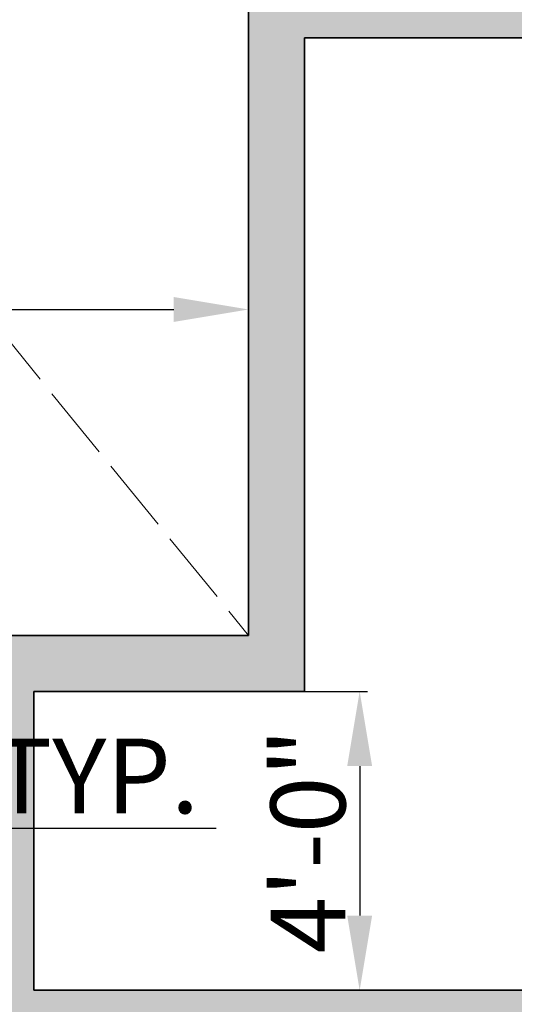
# Model space of a CAD drawing. Units: inches. Extents: x 2083 to 3317, y 1141 to 2115.
# Tile 88 of 256: x 2382 to 2462, y 1419 to 1577. Entities that reach past the tile are written whole.
import ezdxf

# ---------------------------------------------------------------- set-up
doc = ezdxf.new("R2010")
doc.units = ezdxf.units.IN
doc.linetypes.add('ACAD_ISO02W100', pattern=[15, 12, -3])
for name, color, linetype, lineweight in [('A-ANNO-DIMS', 2, 'Continuous', 18), ('A-FLOR-OPEN', 8, 'ACAD_ISO02W100', 13), ('A-WALL', 7, 'Continuous', 35)]:
    doc.layers.add(name, color=color, linetype=linetype, lineweight=lineweight)
doc.layers.add('A-WALL-PATT', color=251, linetype='Continuous', lineweight=13, true_color=0x636466)
doc.styles.get("Standard").update_dxf_attribs({"font": 'arial.ttf'})
doc.dimstyles.new('ISO-25', dxfattribs={"dimtxt": 12, "dimasz": 12, "dimexe": 1.25, "dimexo": 0.625, "dimtad": 1, "dimlunit": 3, "dimtxsty": 'Standard', "dimcen": 2.5, "dimadec": 0, "dimazin": 0, "dimtfac": 1, "dimtmove": 0, "dimatfit": 3, "dimfxl": 1, "dimarcsym": 0})

# ---------------------------------------------------------------- blocks, each defined once
blk = doc.blocks.new('*D30')
at = {"layer": 'A-ANNO-DIMS', "color": 0, "lineweight": -2, "transparency": 16777216}
for p, q in [((2240.02, 1445.27), (2240.02, 1448.05)), ((2254.33, 1445.27), (2254.33, 1448.05)), ((2228.02, 1446.8), (2216.02, 1446.8)), ((2240.02, 1446.8), (2254.33, 1446.8)), ((2266.33, 1446.8), (2413.76, 1446.8))]:
    blk.add_line(p, q, dxfattribs=at)
at = {"layer": 'A-ANNO-DIMS', "color": 0, "transparency": 16777216}
for points in [[(2228.02, 1448.8), (2228.02, 1444.8), (2240.02, 1446.8)], [(2266.33, 1448.8), (2266.33, 1444.8), (2254.33, 1446.8)]]:
    blk.add_solid(points, dxfattribs=at)
at = {"layer": 'Defpoints', "color": 0, "transparency": 16777216}
for p in [(2254.33, 1446.8), (2240.02, 1444.65), (2254.33, 1444.65)]:
    blk.add_point(p, dxfattribs=at)
at = {"layer": 'A-ANNO-DIMS', "color": 0, "transparency": 16777216, "insert": (2346.05, 1453.63), "char_height": 12, "attachment_point": 5}
blk.add_mtext('WC 1\'-2 1/2" TYP.', dxfattribs=at)
blk = doc.blocks.new('*D45')
at = {"layer": 'A-ANNO-DIMS', "color": 0, "lineweight": -2, "transparency": 16777216}
for p, q in [((2235.96, 1478.39), (2235.96, 1531.36)), ((2418.96, 1478.39), (2418.96, 1531.36)), ((2247.96, 1530.11), (2406.96, 1530.11))]:
    blk.add_line(p, q, dxfattribs=at)
at = {"layer": 'A-ANNO-DIMS', "color": 0, "transparency": 16777216}
for points in [[(2247.96, 1532.11), (2247.96, 1528.11), (2235.96, 1530.11)], [(2406.96, 1532.11), (2406.96, 1528.11), (2418.96, 1530.11)]]:
    blk.add_solid(points, dxfattribs=at)
at = {"layer": 'Defpoints', "color": 0, "transparency": 16777216}
for p in [(2418.96, 1530.11), (2235.96, 1477.76), (2418.96, 1477.76)]:
    blk.add_point(p, dxfattribs=at)
at = {"layer": 'A-ANNO-DIMS', "color": 0, "transparency": 16777216, "insert": (2327.46, 1536.87), "char_height": 12, "attachment_point": 5}
blk.add_mtext('15\'-3"', dxfattribs=at)
blk = doc.blocks.new('*D63')
at = {"layer": 'A-ANNO-DIMS', "color": 0, "lineweight": -2, "transparency": 16777216}
for p, q in [((2385.08, 1468.76), (2438.06, 1468.76)), ((2436.81, 1456.76), (2436.81, 1432.76)), ((2385.08, 1420.76), (2438.06, 1420.76))]:
    blk.add_line(p, q, dxfattribs=at)
at = {"layer": 'A-ANNO-DIMS', "color": 0, "transparency": 16777216}
for points in [[(2434.81, 1456.76), (2438.81, 1456.76), (2436.81, 1468.76)], [(2434.81, 1432.76), (2438.81, 1432.76), (2436.81, 1420.76)]]:
    blk.add_solid(points, dxfattribs=at)
at = {"layer": 'Defpoints', "color": 0, "transparency": 16777216}
for p in [(2384.46, 1468.76), (2384.46, 1420.76), (2436.81, 1420.76)]:
    blk.add_point(p, dxfattribs=at)
at = {"layer": 'A-ANNO-DIMS', "color": 0, "transparency": 16777216, "insert": (2430.06, 1444.76), "char_height": 12, "attachment_point": 5, "rotation": 90}
blk.add_mtext('4\'-0"', dxfattribs=at)

msp = doc.modelspace()

# ---------------------------------------------------------------- hatches: boundary and pattern name
at = {"layer": 'A-WALL-PATT'}
h = msp.add_hatch(color=256, dxfattribs=at)
h.dxf.hatch_style = 1
h.paths.add_polyline_path([(3126.96, 2020.761), (2748.96, 2020.761), (2604.96, 2020.761), (2226.96, 2020.761), (2226.96, 1702.761), (2466.96, 1702.761), (2466.96, 1582.761), (2418.96, 1582.761), (2418.96, 1477.761), (2226.96, 1477.761), (2226.96, 1263.261), (2544.96, 1263.261), (2544.96, 1411.761), (2604.96, 1411.761), (2685.96, 1411.761), (2685.96, 1420.761), (2604.96, 1420.761), (2604.96, 1573.761), (2604.96, 1702.761), (2604.96, 2011.761), (2748.96, 2011.761), (2748.96, 1702.761), (2862.96, 1702.761), (2862.96, 1621.761), (2871.96, 1621.761), (2871.96, 1702.761), (2883.96, 1702.761), (2883.96, 1706.939, -0.0264593), (2883.96, 1711.761), (2757.96, 1711.761), (2757.96, 1807.761), (2787.96, 1807.761), (2787.96, 1812.261), (2757.96, 1812.261), (2757.96, 2011.761), (2877.96, 2011.761), (2877.96, 1812.261), (2847.96, 1812.261), (2847.96, 1807.761), (2889.836, 1807.761), (2889.836, 1812.261), (2882.46, 1812.261), (2882.46, 2011.761), (3117.96, 2011.761), (3117.96, 1812.261), (2937.836, 1812.261), (2937.836, 1807.761), (2995.71, 1807.761), (2995.71, 1796.118), (3000.21, 1796.118), (3000.21, 1807.761), (3117.96, 1807.761), (3117.96, 1711.761), (3000.21, 1711.761), (3000.21, 1760.118), (2998.573, 1760.118, -0.020711), (2995.71, 1760.118), (2995.71, 1711.761), (2931.96, 1711.761), (2931.96, 1702.761), (3126.96, 1702.761)])
h.paths.add_polyline_path([(2471.46, 2011.761), (2471.46, 1810.011), (2462.717, 1810.011), (2462.717, 1805.511), (2505.96, 1805.511), (2505.96, 1810.011), (2475.96, 1810.011), (2475.96, 2011.761), (2595.96, 2011.761), (2595.96, 1810.011), (2565.96, 1810.011), (2565.96, 1805.511), (2595.96, 1805.511), (2595.96, 1711.761), (2235.96, 1711.761), (2235.96, 1805.511), (2353.71, 1805.511), (2353.71, 1796.054), (2358.21, 1796.054), (2358.21, 1805.511), (2414.717, 1805.511), (2414.717, 1810.011), (2235.96, 1810.011), (2235.96, 2011.761)], flags=16)
h.paths.add_polyline_path([(2270.205, 1994.61), (2270.205, 1970.61), (2246.205, 1970.61), (2246.205, 1994.61)], flags=0)
edge = h.paths.add_edge_path(flags=0)
edge.add_ellipse((2332.027, 1899.798), major_axis=(-3.043, 3.043), ratio=0.1682525, start_angle=-161.33217, end_angle=-156.30711, ccw=False)
edge.add_ellipse((2333.082, 1898.744), major_axis=(-1.055, 1.055), ratio=0.4535321, start_angle=-123.37102, end_angle=-94.15911)
edge = h.paths.add_edge_path(flags=0)
edge.add_ellipse((2332.027, 1968.876), major_axis=(3.043, 3.043), ratio=0.1682525, start_angle=18.66783, end_angle=23.69289)
edge.add_spline(control_points=[(2332.926, 1970.691), (2332.227, 1970.336), (2330.894, 1969.659), (2328.413, 1970.932), (2327.204, 1967.749), (2324.71, 1969.956), (2322.533, 1967.012), (2320.013, 1971.296), (2317.68, 1968.158), (2316.041, 1967.102), (2315.427, 1966.81)], knot_values=[0, 0, 0, 0, 2.2670587, 4.3245589, 6.6855835, 8.8786411, 11.121502, 14.300359, 17.7552837, 19.732645, 19.732645, 19.732645, 19.732645], degree=3, periodic=0)
edge.add_ellipse((2332.027, 1968.876), major_axis=(3.043, 3.043), ratio=0.1682525, start_angle=18.66783, end_angle=23.69289, ccw=False)
edge.add_ellipse((2333.082, 1969.931), major_axis=(1.055, 1.055), ratio=0.4535321, start_angle=56.62898, end_angle=85.84089, ccw=False)
edge = h.paths.add_edge_path(flags=0)
edge.add_spline(control_points=[(2296.428, 1967.988), (2293.628, 1965.336), (2287.704, 1959.727), (2299.744, 1949.996), (2294.533, 1935.669), (2290.573, 1920.604), (2293.394, 1909.974), (2296.185, 1904.967)], knot_values=[0.0991853, 0.0991853, 0.0991853, 0.0991853, 0.3453009, 0.6198217, 0.9826526, 1.3860932, 1.8105546, 1.8105546, 1.8105546, 1.8105546], degree=3, periodic=0)
edge.add_spline(control_points=[(2296.185, 1904.967), (2297.384, 1902.619), (2298.001, 1901.949), (2298.553, 1901.468)], knot_values=[0.0062457, 0.0062457, 0.0062457, 0.0062457, 0.0554759, 0.0554759, 0.0554759, 0.0554759], degree=3, periodic=0)
edge.add_spline(control_points=[(2298.553, 1901.468), (2297.259, 1900.923), (2295.225, 1900.232), (2293.06, 1900.614), (2292.101, 1900.788), (2292.09, 1900.791)], knot_values=[0.3128349, 0.3128349, 0.3128349, 0.3128349, 0.4017797, 0.4749867, 0.4759027, 0.4759027, 0.4759027, 0.4759027], degree=3, periodic=0)
edge.add_arc((2292.794, 1904.664), 3.937, 215.4209, 259.69818, ccw=False)
edge.add_spline(control_points=[(2289.585, 1902.382), (2289.477, 1902.535), (2289.368, 1902.688), (2289.261, 1902.841)], knot_values=[0.1028719, 0.1028719, 0.1028719, 0.1028719, 0.1168958, 0.1168958, 0.1168958, 0.1168958], degree=3, periodic=0)
edge.add_spline(control_points=[(2289.261, 1902.841), (2288.687, 1902.55), (2287.64, 1902.02), (2285.881, 1901.874), (2283.853, 1901.504), (2281.72, 1899.711), (2278.467, 1899.493), (2276.157, 1901.883), (2272.259, 1899.804), (2267.778, 1901.843), (2262.244, 1900.184), (2257.415, 1901.782), (2254.318, 1900.726), (2253.178, 1900.337)], knot_values=[0, 0, 0, 0, 1.9079767, 3.4771759, 5.261074, 7.9728515, 11.6802485, 13.7179214, 16.9395917, 22.789562, 27.5025027, 33.5952153, 37.1456181, 37.1456181, 37.1456181, 37.1456181], degree=3, periodic=0)
edge.add_line((2253.178, 1900.337), (2250.244, 1902.841))
edge.add_line((2250.244, 1902.841), (2250.244, 1965.833))
edge.add_line((2250.244, 1965.833), (2253.178, 1968.337))
edge.add_spline(control_points=[(2253.178, 1968.337), (2254.318, 1967.948), (2257.415, 1966.892), (2262.244, 1968.49), (2267.778, 1966.831), (2271.527, 1968.537), (2273.876, 1967.828), (2274.207, 1967.728)], knot_values=[0, 0, 0, 0, 0.0901802, 0.2449351, 0.3646438, 0.5132331, 0.5378548, 0.5378548, 0.5378548, 0.5378548], degree=3, periodic=0)
edge.add_arc((2274.353, 1963.793), 3.937, 72.05113, 92.12795, ccw=False)
edge.add_arc((2281.297, 1985.23), 18.596, 252.05113, 288.56572)
edge.add_arc((2292.317, 1956.029), 12.646, 71.02679, 113.77822, ccw=False)
edge = h.paths.add_edge_path(flags=0)
edge.add_spline(control_points=[(2274.899, 1951.856), (2275.066, 1951.617), (2275.233, 1951.377), (2275.398, 1951.136)], knot_values=[1.4099157, 1.4099157, 1.4099157, 1.4099157, 1.4315903, 1.4315903, 1.4315903, 1.4315903], degree=3, periodic=0)
edge.add_spline(control_points=[(2275.398, 1951.136), (2275.792, 1950.562), (2276.179, 1949.984), (2276.546, 1949.397)], knot_values=[1.3582378, 1.3582378, 1.3582378, 1.3582378, 1.4099157, 1.4099157, 1.4099157, 1.4099157], degree=3, periodic=0)
edge.add_line((2276.546, 1949.397), (2277.437, 1947.862))
edge.add_spline(control_points=[(2277.437, 1947.862), (2276.304, 1945.673), (2274.64, 1942.427), (2274.632, 1938.094), (2272.799, 1930.852), (2274.356, 1943.897), (2275.948, 1947.923), (2276.546, 1949.397)], knot_values=[0.0056315, 0.0056315, 0.0056315, 0.0056315, 0.1860139, 0.2660015, 0.3570872, 0.5963902, 0.7397317, 0.7397317, 0.7397317, 0.7397317], degree=3, periodic=0)
edge.add_spline(control_points=[(2276.546, 1949.397), (2276.179, 1949.984), (2275.792, 1950.562), (2275.398, 1951.136)], knot_values=[1.3582378, 1.3582378, 1.3582378, 1.3582378, 1.4099157, 1.4099157, 1.4099157, 1.4099157], degree=3, periodic=0)
edge.add_spline(control_points=[(2275.398, 1951.136), (2274.943, 1950.08), (2274.208, 1948.025), (2273.935, 1944.851), (2272.469, 1937.627), (2273.466, 1945.696), (2274.701, 1951.059), (2274.899, 1951.856)], knot_values=[0.1043639, 0.1043639, 0.1043639, 0.1043639, 0.1896363, 0.2696239, 0.3607096, 0.6000126, 0.6446217, 0.6446217, 0.6446217, 0.6446217], degree=3, periodic=0)
h.paths.add_polyline_path([(2269.168, 1963.128, -0.3575267), (2268.171, 1960.976, -0.0925607), (2268.171, 1939.436, -0.3575267), (2269.168, 1937.285, -0.3575267), (2267.016, 1938.282, -0.1647847), (2254.686, 1938.282, -0.3575267), (2252.534, 1937.285, -0.3575267), (2253.531, 1939.436, -0.0925607), (2253.531, 1960.976, -0.3575267), (2252.534, 1963.128, -0.3575267), (2254.686, 1962.131, -0.1647847), (2267.016, 1962.131, -0.3575267)], flags=0)
h.paths.add_polyline_path([(2248.874, 1967.802), (2248.874, 1957.028), (2249.458, 1957.028), (2249.458, 1911.647), (2248.874, 1911.647), (2248.874, 1900.873), (2246.512, 1900.873, 0.1973271), (2244.15, 1902.457), (2244.15, 1966.218, 0.1973271), (2246.512, 1967.802)], flags=0)
h.paths.add_polyline_path([(2269.168, 1931.389, -0.3575267), (2268.171, 1929.238, -0.0925607), (2268.171, 1907.698, -0.3575267), (2269.168, 1905.547, -0.3575267), (2267.016, 1906.544, -0.1647847), (2254.686, 1906.544, -0.3575267), (2252.534, 1905.547, -0.3575267), (2253.531, 1907.698, -0.0925607), (2253.531, 1929.238, -0.3575267), (2252.534, 1931.389, -0.3575267), (2254.686, 1930.392, -0.1647847), (2267.016, 1930.392, -0.3575267)], flags=0)
edge = h.paths.add_edge_path(flags=0)
edge.add_spline(control_points=[(2276.197, 1906.724), (2276.168, 1909.029), (2276.114, 1913.372), (2270.598, 1924.925), (2273.905, 1919.013), (2275.922, 1916.262), (2275.475, 1912.402), (2277.258, 1910.381), (2276.696, 1908.225), (2276.646, 1906.813), (2276.618, 1906.008)], knot_values=[0, 0, 0, 0, 8.6102597, 16.2212739, 18.8430575, 23.8048978, 27.4408283, 29.3561016, 31.2034776, 33.6506866, 33.6506866, 33.6506866, 33.6506866], degree=3, periodic=0)
edge.add_spline(control_points=[(2276.618, 1906.008), (2276.623, 1905.624), (2276.498, 1904.629), (2275.442, 1903.855), (2274.937, 1903.08), (2274.859, 1902.841)], knot_values=[0.1564884, 0.1564884, 0.1564884, 0.1564884, 0.1843975, 0.2313765, 0.2505985, 0.2505985, 0.2505985, 0.2505985], degree=3, periodic=0)
edge.add_line((2274.859, 1902.841), (2276.506, 1902.841))
edge.add_spline(control_points=[(2276.506, 1902.841), (2276.788, 1903.085), (2277.665, 1904.125), (2278.25, 1904.341), (2277.654, 1908.527), (2278.156, 1906.228), (2278.1, 1905.286), (2278.847, 1904.069), (2277.857, 1903.415), (2277.874, 1902.991), (2277.904, 1902.841)], knot_values=[0.0595743, 0.0595743, 0.0595743, 0.0595743, 0.0807529, 0.1037415, 0.1697201, 0.1760361, 0.2071372, 0.2404744, 0.2623409, 0.2736605, 0.2736605, 0.2736605, 0.2736605], degree=3, periodic=0)
edge.add_line((2277.904, 1902.841), (2280.03, 1902.841))
edge.add_spline(control_points=[(2280.03, 1902.841), (2279.888, 1903.088), (2279.499, 1903.982), (2280.152, 1905.939), (2278.104, 1909.658), (2279.762, 1907.185), (2280.328, 1904.875), (2280.485, 1903.49), (2281.463, 1903.249), (2281.758, 1902.936), (2281.834, 1902.841)], knot_values=[0.013856, 0.013856, 0.013856, 0.013856, 0.0348738, 0.0888667, 0.1078792, 0.1267378, 0.158714, 0.1937575, 0.2174868, 0.2267221, 0.2267221, 0.2267221, 0.2267221], degree=3, periodic=0)
edge.add_spline(control_points=[(2281.834, 1902.841), (2281.788, 1902.827), (2281.647, 1902.783), (2281.396, 1902.859), (2281.088, 1902.985), (2280.721, 1903.061), (2280.333, 1903.026), (2280.125, 1902.899), (2280.03, 1902.841)], knot_values=[0, 0, 0, 0, 0.1441304, 0.435517, 0.7492759, 1.1530457, 1.5483707, 1.878348, 1.878348, 1.878348, 1.878348], degree=3, periodic=0)
edge.add_line((2280.03, 1902.841), (2277.904, 1902.841))
edge.add_spline(control_points=[(2277.904, 1902.841), (2277.893, 1902.796), (2277.865, 1902.68), (2277.607, 1902.687), (2277.274, 1902.801), (2276.838, 1902.62), (2276.584, 1902.789), (2276.506, 1902.841)], knot_values=[0, 0, 0, 0, 0.1271885, 0.3261988, 0.6280094, 1.2435704, 1.5153306, 1.5153306, 1.5153306, 1.5153306], degree=3, periodic=0)
edge.add_line((2276.506, 1902.841), (2274.859, 1902.841))
edge.add_spline(control_points=[(2274.859, 1902.841), (2274.814, 1902.899), (2274.725, 1903.013), (2274.493, 1903.119), (2274.244, 1902.961), (2273.937, 1903.185), (2273.614, 1902.983), (2273.408, 1902.883), (2273.322, 1902.841)], knot_values=[0, 0, 0, 0, 0.2184302, 0.4369566, 0.6879766, 0.9903786, 1.3983955, 1.6918498, 1.6918498, 1.6918498, 1.6918498], degree=3, periodic=0)
edge.add_spline(control_points=[(2273.322, 1902.841), (2273.617, 1903.446), (2274.274, 1904.538), (2276.027, 1904.574), (2276.207, 1906.584), (2276.197, 1906.724)], knot_values=[0.0122268, 0.0122268, 0.0122268, 0.0122268, 0.0594721, 0.1062177, 0.134458, 0.134458, 0.134458, 0.134458], degree=3, periodic=0)
h.paths.add_polyline_path([(2270.776, 1897.79), (2270.776, 1873.79), (2246.776, 1873.79), (2246.776, 1897.79)], flags=0)
h.paths.add_polyline_path([(2353.71, 1760.005), (2353.71, 1760.054), (2358.21, 1760.054, -0.033729)], flags=0)
h.paths.add_polyline_path([(2321.819, 1737.529), (2341.995, 1737.529, -0.4142136), (2343.203, 1736.321), (2343.203, 1721.021, -0.4142136), (2341.995, 1719.813), (2321.819, 1719.813, -0.4142136), (2320.611, 1721.021), (2320.611, 1736.321, -0.4142136)], flags=0)
h.paths.add_polyline_path([(2324.235, 1736.321), (2339.579, 1736.321, -0.4142136), (2341.995, 1733.905), (2341.995, 1725.45, -0.4142136), (2339.579, 1723.034), (2333.681, 1723.034), (2333.845, 1722.045, -0.8706461), (2335.425, 1721.826, -0.767327), (2333.923, 1721.423), (2331.291, 1721.423, -0.767327), (2329.788, 1721.826, -0.8706461), (2331.368, 1722.045), (2331.533, 1723.034), (2324.235, 1723.034, -0.4142136), (2321.819, 1725.45), (2321.819, 1733.905, -0.4142136)], flags=0)
h.paths.add_polyline_path([(2570.484, 1928.615), (2589.684, 1928.615), (2590.169, 1928.615), (2590.169, 1904.993), (2570.484, 1904.993)], flags=0)
h.paths.add_polyline_path([(2574.447, 1927.264, -1), (2572.829, 1927.264, -1)], flags=0)
h.paths.add_polyline_path([(2573.09, 1926.941), (2573.925, 1927.776), (2574.148, 1927.553), (2573.313, 1926.718)], flags=0)
h.paths.add_polyline_path([(2578.779, 1919.73, -1), (2571.592, 1919.73, -1)], flags=0)
h.paths.add_polyline_path([(2578.385, 1919.73, -1), (2571.985, 1919.73, -1)], flags=0)
h.paths.add_polyline_path([(2331.596, 1729.476, -1), (2333.618, 1729.476, -1)], flags=0)
h.paths.add_polyline_path([(2578.034, 1927.264, -1), (2576.416, 1927.264, -1)], flags=0)
h.paths.add_polyline_path([(2576.689, 1927.531), (2576.912, 1927.754), (2577.747, 1926.919), (2577.524, 1926.696)], flags=0)
h.paths.add_polyline_path([(2578.139, 1909.86, -1), (2572.232, 1909.86, -1)], flags=0)
h.paths.add_polyline_path([(2577.745, 1909.86, -1), (2572.625, 1909.86, -1)], flags=0)
h.paths.add_polyline_path([(2583.798, 1927.264, -1), (2582.179, 1927.264, -1)], flags=0)
h.paths.add_polyline_path([(2582.719, 1927.754), (2583.554, 1926.919), (2583.331, 1926.696), (2582.496, 1927.531)], flags=0)
h.paths.add_polyline_path([(2582.496, 1927.531), (2582.719, 1927.754), (2583.554, 1926.919), (2583.331, 1926.696)], flags=0)
h.paths.add_polyline_path([(2587.739, 1920.53, -1), (2581.832, 1920.53, -1)], flags=0)
h.paths.add_polyline_path([(2587.345, 1920.53, -1), (2582.225, 1920.53, -1)], flags=0)
h.paths.add_polyline_path([(2587.385, 1927.264, -1), (2585.766, 1927.264, -1)], flags=0)
h.paths.add_polyline_path([(2586.082, 1926.98), (2586.917, 1927.815), (2587.14, 1927.593), (2586.305, 1926.758)], flags=0)
h.paths.add_polyline_path([(2588.379, 1910.66, -1), (2581.192, 1910.66, -1)], flags=0)
h.paths.add_polyline_path([(2587.985, 1910.66, -1), (2581.585, 1910.66, -1)], flags=0)
h.paths.add_polyline_path([(2417.168, 1729.478), (2437.344, 1729.478, -0.4142136), (2438.552, 1728.27), (2438.552, 1712.969, -0.4142136), (2437.344, 1711.761), (2417.168, 1711.761, -0.4142136), (2415.96, 1712.969), (2415.96, 1728.27, -0.4142136)], flags=0)
h.paths.add_polyline_path([(2419.584, 1728.27), (2434.928, 1728.27, -0.4142136), (2437.344, 1725.854), (2437.344, 1717.398, -0.4142136), (2434.928, 1714.983), (2429.029, 1714.983), (2429.194, 1713.994, -0.8706461), (2430.774, 1713.775, -0.767327), (2429.271, 1713.372), (2426.64, 1713.372, -0.767327), (2425.137, 1713.775, -0.8706461), (2426.717, 1713.994), (2426.882, 1714.983), (2419.584, 1714.983, -0.4142136), (2417.168, 1717.398), (2417.168, 1725.854, -0.4142136)], flags=0)
h.paths.add_polyline_path([(2419.584, 1728.27), (2434.928, 1728.27, -0.4142136), (2437.344, 1725.854), (2437.344, 1717.398, -0.4142136), (2434.928, 1714.983), (2429.029, 1714.983), (2428.358, 1719.009), (2427.553, 1719.009), (2426.882, 1714.983), (2419.584, 1714.983, -0.4142136), (2417.168, 1717.398), (2417.168, 1725.854, -0.4142136)], flags=0)
h.paths.add_polyline_path([(2426.944, 1721.425, -1), (2428.967, 1721.425, -1)], flags=0)
h.paths.add_polyline_path([(2475.96, 1702.761), (2595.96, 1702.761), (2595.96, 1582.761), (2475.96, 1582.761)], flags=16)
h.paths.add_polyline_path([(2427.96, 1573.761), (2595.96, 1573.761), (2595.96, 1468.761), (2595.96, 1420.761), (2384.46, 1420.761), (2384.46, 1468.761), (2427.96, 1468.761)], flags=16)
h.paths.add_polyline_path([(2379.96, 1468.761), (2379.96, 1420.761), (2235.96, 1420.761), (2235.96, 1468.761)], flags=16)
h.paths.add_polyline_path([(2317.816, 1466.696), (2337.992, 1466.696, -0.4142136), (2339.2, 1465.488), (2339.2, 1450.187, -0.4142136), (2337.992, 1448.979), (2317.816, 1448.979, -0.4142136), (2316.608, 1450.187), (2316.608, 1465.488, -0.4142136)], flags=0)
h.paths.add_polyline_path([(2320.232, 1465.488), (2335.576, 1465.488, -0.4142136), (2337.992, 1463.072), (2337.992, 1454.616, -0.4142136), (2335.576, 1452.2), (2329.677, 1452.2), (2329.842, 1451.212, -0.8706461), (2331.422, 1450.992, -0.767327), (2329.92, 1450.59), (2327.288, 1450.59, -0.767327), (2325.785, 1450.992, -0.8706461), (2327.365, 1451.212), (2327.53, 1452.2), (2320.232, 1452.2, -0.4142136), (2317.816, 1454.616), (2317.816, 1463.072, -0.4142136)], flags=0)
h.paths.add_polyline_path([(2320.232, 1465.488), (2335.576, 1465.488, -0.4142136), (2337.992, 1463.072), (2337.992, 1454.616, -0.4142136), (2335.576, 1452.2), (2329.677, 1452.2), (2329.006, 1456.227), (2328.201, 1456.227), (2327.53, 1452.2), (2320.232, 1452.2, -0.4142136), (2317.816, 1454.616), (2317.816, 1463.072, -0.4142136)], flags=0)
h.paths.add_polyline_path([(2327.593, 1458.643, -1), (2329.615, 1458.643, -1)], flags=0)
h.paths.add_polyline_path([(2244.412, 1433.34), (2241.921, 1433.34, -0.4142136), (2240.018, 1435.244), (2240.018, 1440.953, -0.4142105), (2241.921, 1442.856), (2244.412, 1442.856, -1.9764724)], flags=0)
h.paths.add_polyline_path([(2245.357, 1434.398, -0.4142136), (2245.357, 1441.799, -2.1440985)], flags=0)
h.paths.add_polyline_path([(2535.96, 1416.261), (2535.96, 1272.261), (2235.96, 1272.261), (2235.96, 1416.261)], flags=16)
h.paths.add_polyline_path([(2260.12, 1384.293), (2260.12, 1362.039), (2237.865, 1362.039), (2237.865, 1384.293)], flags=0)
edge = h.paths.add_edge_path(flags=0)
edge.add_line((2318.252, 1362.093), (2318.146, 1362.001))
edge.add_ellipse((2317.445, 1360.431), major_axis=(2.822, 2.822), ratio=0.1682525, start_angle=18.66783, end_angle=20.94813, ccw=False)
edge.add_ellipse((2318.423, 1361.409), major_axis=(0.978, 0.978), ratio=0.4535321, start_angle=56.62898, end_angle=70.2262, ccw=False)
edge = h.paths.add_edge_path(flags=0)
edge.add_line((2319.107, 1295.571), (2319.015, 1295.677))
edge.add_ellipse((2317.445, 1296.378), major_axis=(-2.822, 2.822), ratio=0.1682525, start_angle=-161.33217, end_angle=-159.05187, ccw=False)
edge.add_ellipse((2318.423, 1295.4), major_axis=(-0.978, 0.978), ratio=0.4535321, start_angle=-123.37102, end_angle=-109.7738)
edge = h.paths.add_edge_path(flags=0)
edge.add_spline(control_points=[(2284.21, 1301.17), (2284.581, 1300.445), (2284.891, 1299.892), (2285.16, 1299.461)], knot_values=[0.0390658, 0.0390658, 0.0390658, 0.0390658, 0.0554759, 0.0554759, 0.0554759, 0.0554759], degree=3, periodic=0)
edge.add_line((2285.16, 1299.461), (2284.21, 1301.17))
edge = h.paths.add_edge_path(flags=0)
edge.add_line((2280.412, 1297.298), (2283.37, 1297.036))
edge.add_line((2283.37, 1297.036), (2286.406, 1297.926))
edge.add_spline(control_points=[(2286.406, 1297.926), (2285.305, 1297.463), (2284.345, 1297.129), (2283.37, 1297.036)], knot_values=[0.3943688, 0.3943688, 0.3943688, 0.3943688, 0.4759027, 0.4759027, 0.4759027, 0.4759027], degree=3, periodic=0)
edge.add_spline(control_points=[(2283.37, 1297.036), (2283.281, 1297.028), (2282.316, 1296.957), (2281.313, 1297.134), (2280.423, 1297.296), (2280.412, 1297.298)], knot_values=[0.3128349, 0.3128349, 0.3128349, 0.3128349, 0.3202458, 0.3934528, 0.3943688, 0.3943688, 0.3943688, 0.3943688], degree=3, periodic=0)
edge = h.paths.add_edge_path(flags=0)
edge.add_line((2284.436, 1359.607), (2280.446, 1355.328))
edge.add_line((2280.446, 1355.328), (2279.58, 1351.018))
edge.add_line((2279.58, 1351.018), (2282.413, 1346.58))
edge.add_spline(control_points=[(2282.413, 1346.58), (2283.153, 1345.589), (2284.253, 1344.029), (2284.801, 1342.387), (2284.935, 1341.806)], knot_values=[1.2400982, 1.2400982, 1.2400982, 1.2400982, 1.3328922, 1.3827123, 1.3827123, 1.3827123, 1.3827123], degree=3, periodic=0)
edge.add_spline(control_points=[(2284.935, 1341.806), (2285.319, 1340.141), (2285.233, 1338.409), (2284.91, 1336.654)], knot_values=[1.0974841, 1.0974841, 1.0974841, 1.0974841, 1.2400982, 1.2400982, 1.2400982, 1.2400982], degree=3, periodic=0)
edge.add_spline(control_points=[(2284.91, 1336.654), (2284.587, 1334.899), (2284.027, 1333.12), (2283.463, 1331.361)], knot_values=[0.9548699, 0.9548699, 0.9548699, 0.9548699, 1.0974841, 1.0974841, 1.0974841, 1.0974841], degree=3, periodic=0)
edge.add_line((2283.463, 1331.361), (2281.89, 1326.153))
edge.add_line((2281.89, 1326.153), (2280.756, 1321.056))
edge.add_line((2280.756, 1321.056), (2280.299, 1316.002))
edge.add_line((2280.299, 1316.002), (2280.716, 1310.95))
edge.add_line((2280.716, 1310.95), (2282.028, 1305.972))
edge.add_line((2282.028, 1305.972), (2284.21, 1301.17))
edge.add_spline(control_points=[(2284.21, 1301.17), (2283.341, 1302.73), (2282.612, 1304.336), (2282.028, 1305.972)], knot_values=[0.0991853, 0.0991853, 0.0991853, 0.0991853, 0.2417994, 0.2417994, 0.2417994, 0.2417994], degree=3, periodic=0)
edge.add_spline(control_points=[(2282.028, 1305.972), (2281.444, 1307.608), (2281.005, 1309.273), (2280.716, 1310.95)], knot_values=[0.2417994, 0.2417994, 0.2417994, 0.2417994, 0.3844135, 0.3844135, 0.3844135, 0.3844135], degree=3, periodic=0)
edge.add_spline(control_points=[(2280.716, 1310.95), (2280.433, 1312.588), (2280.289, 1314.277), (2280.299, 1315.962), (2280.299, 1316.002)], knot_values=[0.3844135, 0.3844135, 0.3844135, 0.3844135, 0.5236467, 0.5270276, 0.5270276, 0.5270276, 0.5270276], degree=3, periodic=0)
edge.add_spline(control_points=[(2280.299, 1316.002), (2280.312, 1317.687), (2280.478, 1319.368), (2280.756, 1321.056)], knot_values=[0.5270276, 0.5270276, 0.5270276, 0.5270276, 0.6696417, 0.6696417, 0.6696417, 0.6696417], degree=3, periodic=0)
edge.add_spline(control_points=[(2280.756, 1321.056), (2281.035, 1322.744), (2281.426, 1324.44), (2281.89, 1326.153)], knot_values=[0.6696417, 0.6696417, 0.6696417, 0.6696417, 0.8122558, 0.8122558, 0.8122558, 0.8122558], degree=3, periodic=0)
edge.add_spline(control_points=[(2281.89, 1326.153), (2282.264, 1327.533), (2282.788, 1329.262), (2283.353, 1331.018), (2283.463, 1331.361)], knot_values=[0.8122558, 0.8122558, 0.8122558, 0.8122558, 0.9270873, 0.9548699, 0.9548699, 0.9548699, 0.9548699], degree=3, periodic=0)
edge.add_line((2283.463, 1331.361), (2284.91, 1336.654))
edge.add_line((2284.91, 1336.654), (2284.935, 1341.806))
edge.add_line((2284.935, 1341.806), (2282.413, 1346.58))
edge.add_spline(control_points=[(2282.413, 1346.58), (2281.275, 1348.104), (2280.078, 1349.57), (2279.58, 1351.018)], knot_values=[1.3827123, 1.3827123, 1.3827123, 1.3827123, 1.5253264, 1.5253264, 1.5253264, 1.5253264], degree=3, periodic=0)
edge.add_spline(control_points=[(2279.58, 1351.018), (2279.443, 1351.415), (2279.136, 1352.857), (2279.735, 1354.29), (2280.446, 1355.328)], knot_values=[1.5253264, 1.5253264, 1.5253264, 1.5253264, 1.564439, 1.6679405, 1.6679405, 1.6679405, 1.6679405], degree=3, periodic=0)
edge.add_spline(control_points=[(2280.446, 1355.328), (2281.426, 1356.758), (2282.931, 1358.183), (2284.436, 1359.607)], knot_values=[1.6679405, 1.6679405, 1.6679405, 1.6679405, 1.8105546, 1.8105546, 1.8105546, 1.8105546], degree=3, periodic=0)
edge.add_arc((2280.623, 1348.518), 11.726, 71.02679, 113.77822)
edge.add_arc((2270.405, 1375.595), 17.244, 252.05113, 288.56572, ccw=False)
edge.add_arc((2263.966, 1355.718), 3.651, 72.05113, 92.12795)
edge.add_arc((2263.966, 1355.718), 3.651, 92.12795, 177.98513)
edge.add_spline(control_points=[(2260.318, 1355.846), (2260.26, 1354.221), (2260.551, 1350.187), (2262.999, 1346.766), (2264.473, 1344.649)], knot_values=[1.4315903, 1.4315903, 1.4315903, 1.4315903, 1.5641438, 1.7706953, 1.7706953, 1.7706953, 1.7706953], degree=3, periodic=0)
edge.add_line((2264.473, 1344.649), (2264.936, 1343.983))
edge.add_spline(control_points=[(2263.801, 1340.248), (2263.843, 1340.514), (2264.067, 1341.756), (2264.513, 1343.002), (2264.935, 1343.981)], knot_values=[0.5365702, 0.5365702, 0.5365702, 0.5365702, 0.5593494, 0.6446217, 0.6446217, 0.6446217, 0.6446217], degree=3, periodic=0)
edge.add_spline(control_points=[(2264.935, 1343.981), (2265.118, 1343.715), (2265.299, 1343.448), (2265.477, 1343.179)], knot_values=[1.3840767, 1.3840767, 1.3840767, 1.3840767, 1.4099157, 1.4099157, 1.4099157, 1.4099157], degree=3, periodic=0)
edge.add_spline(control_points=[(2265.477, 1343.179), (2265.655, 1342.911), (2265.829, 1342.641), (2265.999, 1342.369)], knot_values=[1.3582378, 1.3582378, 1.3582378, 1.3582378, 1.3840767, 1.3840767, 1.3840767, 1.3840767], degree=3, periodic=0)
edge.add_line((2265.999, 1342.369), (2266.826, 1340.946))
edge.add_spline(control_points=[(2266.826, 1340.946), (2268.894, 1337.09), (2271.398, 1325.843), (2270.516, 1310.569), (2275.919, 1301.861), (2277.79, 1299.199)], knot_values=[0.1168958, 0.1168958, 0.1168958, 0.1168958, 0.4729873, 1.0509689, 1.3137934, 1.3137934, 1.3137934, 1.3137934], degree=3, periodic=0)
edge.add_spline(control_points=[(2277.79, 1299.199), (2277.839, 1299.128), (2277.889, 1299.057), (2277.94, 1298.987)], knot_values=[0.1098839, 0.1098839, 0.1098839, 0.1098839, 0.1168958, 0.1168958, 0.1168958, 0.1168958], degree=3, periodic=0)
edge.add_line((2277.94, 1298.987), (2277.789, 1299.199))
edge.add_spline(control_points=[(2277.789, 1299.199), (2277.257, 1298.929), (2276.286, 1298.438), (2275.039, 1298.334), (2274.383, 1298.239), (2274.215, 1298.209)], knot_values=[33.1218702, 33.1218702, 33.1218702, 33.1218702, 35.0290557, 36.5982549, 37.1448269, 37.1448269, 37.1448269, 37.1448269], degree=3, periodic=0)
edge.add_line((2274.215, 1298.209), (2273.073, 1297.893))
edge.add_spline(control_points=[(2273.073, 1297.893), (2272.323, 1297.58), (2271.039, 1296.511), (2269.248, 1296.226), (2268.423, 1296.375)], knot_values=[26.5325843, 26.5325843, 26.5325843, 26.5325843, 29.198919, 31.8391012, 31.8391012, 31.8391012, 31.8391012], degree=3, periodic=0)
edge.add_line((2268.423, 1296.375), (2263.879, 1297.458))
edge.add_spline(control_points=[(2263.879, 1297.458), (2263.556, 1297.359), (2261.86, 1296.839), (2260.239, 1297.282), (2258.933, 1297.516)], knot_values=[15.9195506, 15.9195506, 15.9195506, 15.9195506, 16.9395917, 21.2260675, 21.2260675, 21.2260675, 21.2260675], degree=3, periodic=0)
edge.add_line((2258.933, 1297.516), (2254.055, 1297.329))
edge.add_spline(control_points=[(2254.055, 1297.329), (2253.756, 1297.296), (2252.114, 1297.165), (2250.462, 1297.544), (2249.13, 1297.668)], knot_values=[5.3065169, 5.3065169, 5.3065169, 5.3065169, 6.2764352, 10.6130337, 10.6130337, 10.6130337, 10.6130337], degree=3, periodic=0)
edge.add_line((2249.13, 1297.668), (2244.332, 1296.878))
edge.add_line((2244.332, 1296.878), (2241.611, 1299.199))
edge.add_line((2241.611, 1299.199), (2241.611, 1357.609))
edge.add_line((2241.611, 1357.609), (2244.332, 1359.931))
edge.add_line((2244.332, 1359.931), (2252.729, 1359.543))
edge.add_spline(control_points=[(2252.729, 1359.543), (2252.871, 1359.546), (2253.306, 1359.548), (2253.74, 1359.514), (2254.032, 1359.482)], knot_values=[0.233291, 0.233291, 0.233291, 0.233291, 0.2449351, 0.2689274, 0.2689274, 0.2689274, 0.2689274], degree=3, periodic=0)
edge.add_line((2254.032, 1359.482), (2259.587, 1359.416))
edge.add_spline(control_points=[(2259.587, 1359.416), (2260.677, 1359.629), (2262.073, 1359.897), (2263.524, 1359.459), (2263.83, 1359.366)], knot_values=[0.4225164, 0.4225164, 0.4225164, 0.4225164, 0.5132331, 0.5378548, 0.5378548, 0.5378548, 0.5378548], degree=3, periodic=0)
edge.add_arc((2263.966, 1355.718), 3.651, 72.05113, 92.12795, ccw=False)
edge.add_arc((2270.405, 1375.595), 17.244, 252.05113, 288.56572)
edge.add_arc((2280.623, 1348.518), 11.726, 71.02679, 113.77822, ccw=False)
h.paths.add_polyline_path([(2240.341, 1359.435), (2240.341, 1349.444), (2240.882, 1349.444), (2240.882, 1307.365), (2240.341, 1307.365), (2240.341, 1297.374), (2238.15, 1297.374, 0.1973271), (2235.96, 1298.843), (2235.96, 1357.966, 0.1973271), (2238.15, 1359.435)], flags=0)
h.paths.add_polyline_path([(2259.158, 1355.101, -0.3575267), (2258.233, 1353.106, -0.0925607), (2258.233, 1333.133, -0.3575267), (2259.158, 1331.138, -0.3575267), (2257.163, 1332.062, -0.1647847), (2245.729, 1332.062, -0.3575267), (2243.735, 1331.138, -0.3575267), (2244.659, 1333.133, -0.0925607), (2244.659, 1353.106, -0.3575267), (2243.735, 1355.101, -0.3575267), (2245.729, 1354.176, -0.1647847), (2257.163, 1354.176, -0.3575267)], flags=0)
edge = h.paths.add_edge_path(flags=0)
edge.add_line((2265.999, 1342.369), (2266.826, 1340.946))
edge.add_line((2266.826, 1340.946), (2265.308, 1337.814))
edge.add_line((2265.308, 1337.814), (2264.358, 1334.653))
edge.add_line((2264.358, 1334.653), (2264.262, 1333.8))
edge.add_spline(control_points=[(2264.262, 1333.8), (2264.208, 1333.187), (2264.162, 1332.366), (2264.007, 1331.414), (2263.969, 1331.202)], knot_values=[0.4644442, 0.4644442, 0.4644442, 0.4644442, 0.5166905, 0.5316081, 0.5316081, 0.5316081, 0.5316081], degree=3, periodic=0)
edge.add_spline(control_points=[(2263.969, 1331.202), (2263.775, 1330.119), (2263.424, 1328.791), (2263.257, 1328.531), (2263.234, 1328.515)], knot_values=[0.3726816, 0.3726816, 0.3726816, 0.3726816, 0.4488497, 0.4644442, 0.4644442, 0.4644442, 0.4644442], degree=3, periodic=0)
edge.add_spline(control_points=[(2263.234, 1328.515), (2263.096, 1328.42), (2263.131, 1329.301), (2263.275, 1330.616)], knot_values=[0.2809191, 0.2809191, 0.2809191, 0.2809191, 0.3726816, 0.3726816, 0.3726816, 0.3726816], degree=3, periodic=0)
edge.add_spline(control_points=[(2263.275, 1330.616), (2263.419, 1331.93), (2263.672, 1333.677), (2263.97, 1335.315)], knot_values=[0.1891566, 0.1891566, 0.1891566, 0.1891566, 0.2809191, 0.2809191, 0.2809191, 0.2809191], degree=3, periodic=0)
edge.add_spline(control_points=[(2263.97, 1335.315), (2264.1, 1336.032), (2264.419, 1337.622), (2264.755, 1338.864), (2264.947, 1339.491)], knot_values=[0.097394, 0.097394, 0.097394, 0.097394, 0.1375775, 0.1891566, 0.1891566, 0.1891566, 0.1891566], degree=3, periodic=0)
edge.add_spline(control_points=[(2264.947, 1339.491), (2265.29, 1340.606), (2265.644, 1341.494), (2265.999, 1342.369)], knot_values=[0.0056315, 0.0056315, 0.0056315, 0.0056315, 0.097394, 0.097394, 0.097394, 0.097394], degree=3, periodic=0)
h.paths.add_polyline_path([(2259.158, 1325.671, -0.3575267), (2258.233, 1323.676, -0.0925607), (2258.233, 1303.703, -0.3575267), (2259.158, 1301.708, -0.3575267), (2257.163, 1302.633, -0.1647847), (2245.729, 1302.633, -0.3575267), (2243.735, 1301.708, -0.3575267), (2244.659, 1303.703, -0.0925607), (2244.659, 1323.676, -0.3575267), (2243.735, 1325.671, -0.3575267), (2245.729, 1324.747, -0.1647847), (2257.163, 1324.747, -0.3575267)], flags=0)
edge = h.paths.add_edge_path(flags=0)
edge.add_spline(control_points=[(2261.709, 1317.311), (2261.679, 1317.418), (2261.762, 1317.389), (2262.491, 1316.09), (2262.962, 1315.301)], knot_values=[14.9558607, 14.9558607, 14.9558607, 14.9558607, 16.2212739, 18.6948259, 18.6948259, 18.6948259, 18.6948259], degree=3, periodic=0)
edge.add_spline(control_points=[(2262.962, 1315.301), (2262.99, 1315.254), (2263.702, 1314.067), (2264.349, 1313.127), (2264.73, 1312.164)], knot_values=[18.6948259, 18.6948259, 18.6948259, 18.6948259, 18.8430575, 22.433791, 22.433791, 22.433791, 22.433791], degree=3, periodic=0)
edge.add_spline(control_points=[(2264.73, 1312.164), (2264.876, 1311.796), (2265.177, 1310.77), (2265.143, 1309.559), (2265.248, 1308.824)], knot_values=[22.433791, 22.433791, 22.433791, 22.433791, 23.8048978, 26.1727562, 26.1727562, 26.1727562, 26.1727562], degree=3, periodic=0)
edge.add_line((2265.248, 1308.824), (2265.851, 1307.172))
edge.add_spline(control_points=[(2265.851, 1307.172), (2266.065, 1306.822), (2266.384, 1306.332), (2266.424, 1305.781), (2266.42, 1305.611)], knot_values=[28.0625624, 28.0625624, 28.0625624, 28.0625624, 29.3561016, 29.9117214, 29.9117214, 29.9117214, 29.9117214], degree=3, periodic=0)
edge.add_spline(control_points=[(2266.42, 1305.611), (2266.416, 1305.433), (2266.394, 1305.25), (2266.365, 1305.066)], knot_values=[29.9117214, 29.9117214, 29.9117214, 29.9117214, 30.4978371, 30.4978371, 30.4978371, 30.4978371], degree=3, periodic=0)
edge.add_line((2266.365, 1305.066), (2266.066, 1302.136))
edge.add_spline(control_points=[(2266.066, 1302.136), (2266.071, 1301.78), (2265.998, 1301.2), (2265.663, 1300.759), (2265.509, 1300.586)], knot_values=[0.1564884, 0.1564884, 0.1564884, 0.1564884, 0.1843975, 0.2035434, 0.2035434, 0.2035434, 0.2035434], degree=3, periodic=0)
edge.add_line((2265.509, 1300.586), (2264.435, 1299.199))
edge.add_line((2264.435, 1299.199), (2265.962, 1299.199))
edge.add_line((2265.962, 1299.199), (2267.336, 1301.175))
edge.add_line((2267.336, 1301.175), (2267.312, 1301.986))
edge.add_spline(control_points=[(2267.312, 1301.986), (2267.261, 1302.862), (2267.16, 1303.737), (2267.271, 1303.326)], knot_values=[0.1262286, 0.1262286, 0.1262286, 0.1262286, 0.1666174, 0.1666174, 0.1666174, 0.1666174], degree=3, periodic=0)
edge.add_spline(control_points=[(2267.271, 1303.326), (2267.28, 1303.294), (2267.31, 1303.175), (2267.373, 1302.884), (2267.406, 1302.683), (2267.418, 1302.601)], knot_values=[0.1666174, 0.1666174, 0.1666174, 0.1666174, 0.1697201, 0.1760361, 0.1807647, 0.1807647, 0.1807647, 0.1807647], degree=3, periodic=0)
edge.add_spline(control_points=[(2267.744, 1300.988), (2267.688, 1301.151), (2267.481, 1301.657), (2267.484, 1302.145), (2267.418, 1302.601)], knot_values=[0.1807647, 0.1807647, 0.1807647, 0.1807647, 0.1937665, 0.2201389, 0.2201389, 0.2201389, 0.2201389], degree=3, periodic=0)
edge.add_line((2267.418, 1302.601), (2267.744, 1300.988))
edge.add_spline(control_points=[(2267.744, 1300.988), (2267.832, 1300.732), (2267.932, 1300.31), (2267.555, 1299.975), (2267.429, 1299.829)], knot_values=[0.2201389, 0.2201389, 0.2201389, 0.2201389, 0.2404744, 0.2548903, 0.2548903, 0.2548903, 0.2548903], degree=3, periodic=0)
edge.add_line((2267.429, 1299.829), (2267.258, 1299.199))
edge.add_line((2267.258, 1299.199), (2269.23, 1299.199))
edge.add_spline(control_points=[(2269.23, 1299.199), (2269.099, 1299.429), (2268.843, 1300.016), (2269.012, 1300.916), (2268.947, 1301.661)], knot_values=[0.013856, 0.013856, 0.013856, 0.013856, 0.0348738, 0.0670726, 0.0670726, 0.0670726, 0.0670726], degree=3, periodic=0)
edge.add_line((2268.947, 1301.661), (2268.432, 1303.603))
edge.add_spline(control_points=[(2268.432, 1303.603), (2268.176, 1304.192), (2267.596, 1305.251), (2268.041, 1304.623), (2268.251, 1304.282)], knot_values=[0.0901547, 0.0901547, 0.0901547, 0.0901547, 0.1078792, 0.1202891, 0.1202891, 0.1202891, 0.1202891], degree=3, periodic=0)
edge.add_spline(control_points=[(2268.251, 1304.282), (2268.361, 1304.105), (2269.058, 1302.918), (2269.383, 1301.59), (2269.521, 1300.776), (2269.575, 1300.556)], knot_values=[0.1202891, 0.1202891, 0.1202891, 0.1202891, 0.1267378, 0.158714, 0.1735056, 0.1735056, 0.1735056, 0.1735056], degree=3, periodic=0)
edge.add_line((2269.575, 1300.556), (2270.686, 1299.421))
edge.add_spline(control_points=[(2270.686, 1299.421), (2270.767, 1299.357), (2270.838, 1299.281), (2270.903, 1299.199)], knot_values=[0.2181597, 0.2181597, 0.2181597, 0.2181597, 0.2267221, 0.2267221, 0.2267221, 0.2267221], degree=3, periodic=0)
edge.add_line((2270.937, 1299.193), (2270.903, 1299.199))
edge.add_spline(control_points=[(2270.903, 1299.199), (2270.86, 1299.186), (2270.73, 1299.146), (2270.496, 1299.216), (2270.272, 1299.308), (2270.121, 1299.348), (2270.063, 1299.36)], knot_values=[0.939174, 0.939174, 0.939174, 0.939174, 1.0833044, 1.3746911, 1.6884499, 1.878348, 1.878348, 1.878348, 1.878348], degree=3, periodic=0)
edge.add_line((2270.063, 1299.36), (2269.23, 1299.199))
edge.add_line((2269.23, 1299.199), (2267.258, 1299.199))
edge.add_spline(control_points=[(2267.258, 1299.199), (2267.248, 1299.157), (2267.223, 1299.05), (2266.984, 1299.057), (2266.809, 1299.116), (2266.677, 1299.109), (2266.637, 1299.105)], knot_values=[0.7576653, 0.7576653, 0.7576653, 0.7576653, 0.8848538, 1.0838641, 1.3856747, 1.5153306, 1.5153306, 1.5153306, 1.5153306], degree=3, periodic=0)
edge.add_spline(control_points=[(2266.637, 1299.105), (2266.485, 1299.089), (2266.236, 1299.017), (2266.035, 1299.151), (2265.962, 1299.199)], knot_values=[0, 0, 0, 0, 0.4859051, 0.7576653, 0.7576653, 0.7576653, 0.7576653], degree=3, periodic=0)
edge.add_line((2265.962, 1299.199), (2264.435, 1299.199))
edge.add_line((2264.435, 1299.199), (2263.858, 1299.367))
edge.add_spline(control_points=[(2263.858, 1299.367), (2263.819, 1299.371), (2263.78, 1299.386), (2263.74, 1299.402)], knot_values=[0.8459249, 0.8459249, 0.8459249, 0.8459249, 0.9786272, 0.9786272, 0.9786272, 0.9786272], degree=3, periodic=0)
edge.add_line((2263.722, 1299.396), (2263.01, 1299.199))
edge.add_spline(control_points=[(2263.01, 1299.199), (2263.246, 1299.683), (2263.506, 1300.128), (2263.873, 1300.408)], knot_values=[0.0122268, 0.0122268, 0.0122268, 0.0122268, 0.0529705, 0.0529705, 0.0529705, 0.0529705], degree=3, periodic=0)
edge.add_spline(control_points=[(2263.873, 1300.408), (2263.932, 1300.453), (2264.084, 1300.553), (2264.255, 1300.624), (2264.36, 1300.665)], knot_values=[0.0529705, 0.0529705, 0.0529705, 0.0529705, 0.0594721, 0.0690861, 0.0690861, 0.0690861, 0.0690861], degree=3, periodic=0)
edge.add_line((2264.36, 1300.665), (2265.142, 1301.078))
edge.add_line((2265.142, 1301.078), (2265.676, 1302.8))
edge.add_line((2265.676, 1302.8), (2265.541, 1305.704))
edge.add_line((2265.541, 1305.704), (2264.803, 1309.328))
edge.add_line((2264.803, 1309.328), (2263.041, 1314.092))
edge.add_spline(control_points=[(2263.041, 1314.092), (2262.384, 1315.671), (2261.796, 1316.998), (2261.709, 1317.311)], knot_values=[11.2168955, 11.2168955, 11.2168955, 11.2168955, 14.9558607, 14.9558607, 14.9558607, 14.9558607], degree=3, periodic=0)
h.paths.add_polyline_path([(2871.96, 1416.261), (2895.91, 1416.261), (2895.91, 1420.761), (2871.96, 1420.761), (2871.96, 1501.761), (2862.96, 1501.761), (2862.96, 1420.761), (2805.96, 1420.761), (2805.96, 1411.761), (2862.96, 1411.761), (2862.96, 1263.261), (3126.96, 1263.261), (3126.96, 1411.761), (3126.96, 1486.761), (2943.96, 1486.761), (2943.96, 1477.761), (2967.86, 1477.761), (2967.86, 1420.761), (2943.91, 1420.761), (2943.91, 1416.261), (3117.96, 1416.261), (3117.96, 1420.761), (2972.36, 1420.761), (2972.36, 1477.761), (3117.96, 1477.761), (3117.96, 1420.761), (3117.96, 1272.261), (2871.96, 1272.261)], flags=0)
h.paths.add_polyline_path([(2457.126, 1485.943), (2527.603, 1485.943), (2527.603, 1537.636), (2457.126, 1537.636)], flags=8)
h.paths.add_polyline_path([(2481.005, 1609.982), (2590.766, 1609.982), (2590.766, 1682.003), (2481.005, 1682.003)], flags=8)
h.paths.add_polyline_path([(2483.085, 1729.127), (2553.562, 1729.127), (2553.562, 1780.82), (2483.085, 1780.82)], flags=8)

# ---------------------------------------------------------------- linework, layer by layer
at = {"layer": 'A-FLOR-OPEN'}
msp.add_line((2235.96, 1702.761), (2418.96, 1477.761), dxfattribs=at)
at = {"layer": 'A-WALL'}
for p, q in [((2418.96, 1702.761), (2418.96, 1477.761)), ((2427.96, 1573.761), (2595.96, 1573.761)), ((2427.96, 1573.761), (2427.96, 1468.761)), ((2427.96, 1573.761), (2595.96, 1573.761)), ((2427.96, 1468.761), (2427.96, 1573.761)), ((2226.96, 1477.761), (2418.96, 1477.761)), ((2384.46, 1468.761), (2384.46, 1420.761)), ((2384.46, 1468.761), (2427.96, 1468.761)), ((2384.46, 1420.761), (2384.46, 1468.761)), ((2384.46, 1468.761), (2427.96, 1468.761)), ((2384.46, 1420.761), (2595.96, 1420.761)), ((2595.96, 1420.761), (2384.46, 1420.761))]:
    msp.add_line(p, q, dxfattribs=at)

# ---------------------------------------------------------------- dimensions: what is measured, and where the dimension line sits
at = {"layer": 'A-ANNO-DIMS'}
dim = msp.add_linear_dim(base=(2418.96, 1530.111), p1=(2235.96, 1477.761), p2=(2418.96, 1477.761), dimstyle='ISO-25', override={"dimdec": 1, "dimlfac": 1, "dimrnd": 0, "dimzin": 1, "dimdsep": 46, "dimlunit": 4, "dimfrac": 2}, dxfattribs=at)
dim.commit()
dim.dimension.update_dxf_attribs({"geometry": '*D45', "text_midpoint": (2327.46, 1536.867)})
dim = msp.add_linear_dim(base=(2254.329, 1446.796), p1=(2240.018, 1444.649), p2=(2254.329, 1444.649), text='WC <> TYP.', dimstyle='ISO-25', override={"dimdec": 1, "dimlfac": 1, "dimrnd": 0, "dimzin": 1, "dimdsep": 46, "dimlunit": 4, "dimfrac": 2}, dxfattribs=at)
dim.commit()
dim.dimension.update_dxf_attribs({"geometry": '*D30', "text_midpoint": (2346.047, 1453.625)})
dim = msp.add_linear_dim(base=(2436.81, 1420.761), p1=(2384.46, 1468.761), p2=(2384.46, 1420.761), angle=270, dimstyle='ISO-25', override={"dimdec": 1, "dimlfac": 1, "dimrnd": 0, "dimzin": 1, "dimdsep": 46, "dimlunit": 4, "dimfrac": 2}, dxfattribs=at)
dim.commit()
dim.dimension.update_dxf_attribs({"geometry": '*D63', "text_midpoint": (2430.058, 1444.761)})

doc.saveas('drawing.dxf')
